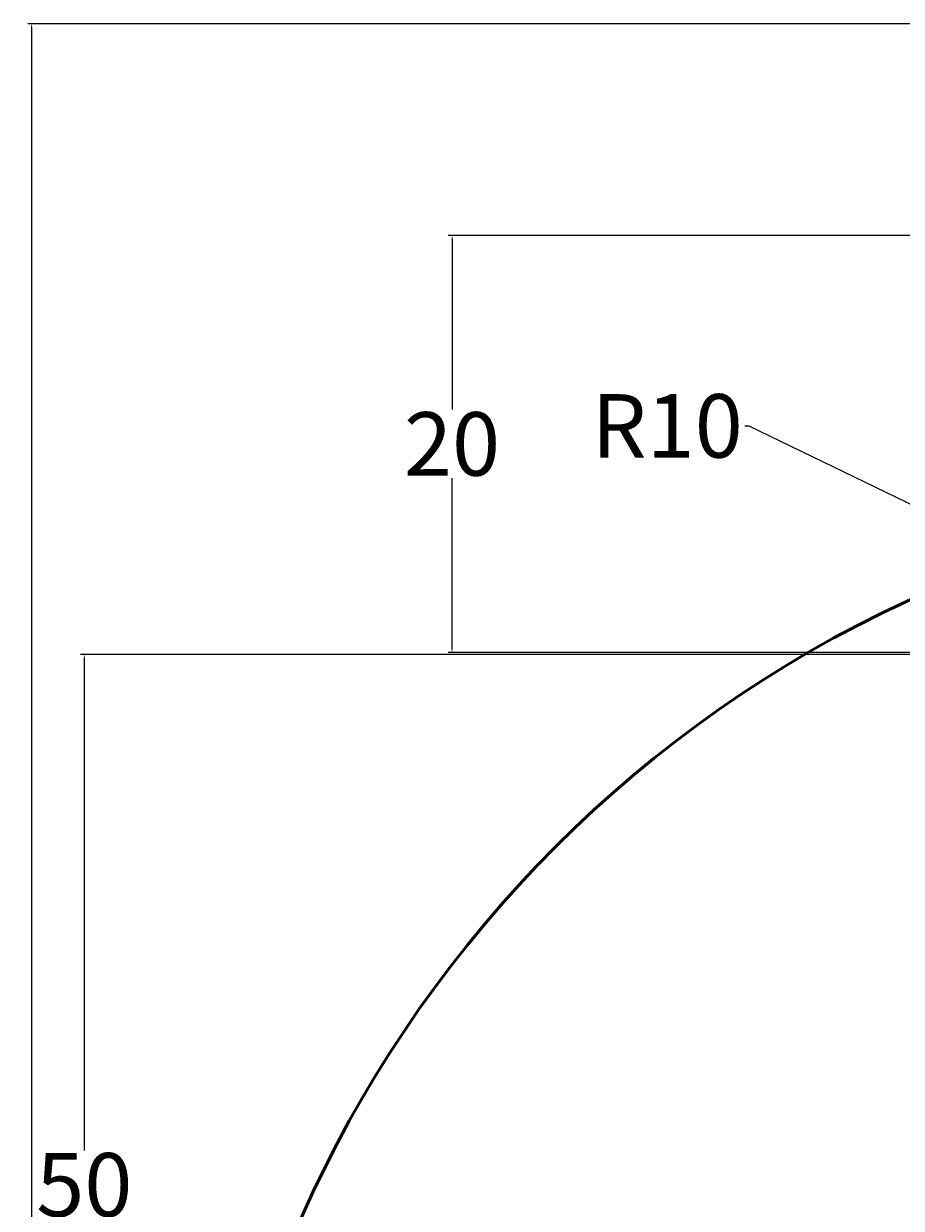
# Model space of a CAD drawing. Units: millimetres. Extents: x -53 to 92, y -147 to 37.
# Tile 10 of 16: x -47 to -6, y -30 to 26. Entities that reach past the tile are written whole.
import ezdxf

# ---------------------------------------------------------------- set-up
doc = ezdxf.new("R2010")
doc.units = ezdxf.units.MM
doc.header["$MEASUREMENT"] = 0
doc.layers.add('M-DIMS', color=2, linetype='Continuous', lineweight=25)
doc.layers.add('M-OUTL', color=7, linetype='Continuous', lineweight=50)
doc.styles.get("Standard").update_dxf_attribs({"font": 'arial.ttf'})
doc.dimstyles.get("Standard").update_dxf_attribs({"dimtxt": 0.18, "dimasz": 0.18, "dimexe": 0.18, "dimexo": 0.0625, "dimgap": 0.09, "dimtad": 0, "dimtih": 1, "dimtoh": 1, "dimdec": 4, "dimzin": 0, "dimdsep": 46, "dimtxsty": 'Standard', "dimcen": 0.09, "dimadec": 0, "dimazin": 0, "dimtfac": 1, "dimtdec": 4, "dimtofl": 0, "dimtmove": 0, "dimatfit": 3, "dimfxl": 1, "dimtolj": 1, "dimtzin": 0, "dimarcsym": 0})

# ---------------------------------------------------------------- blocks, each defined once
blk = doc.blocks.new('*D2')
at = {"layer": 'Defpoints', "color": 0, "transparency": 16777216}
for p in [(0.354, 0.478), (9.355, -3.88)]:
    blk.add_point(p, dxfattribs=at)
at = {"layer": 'M-DIMS', "color": 0, "lineweight": -2, "transparency": 16777216}
for p, q in [((-13.114, 6.912), (-12.934, 6.912)), ((-12.934, 6.912), (0.192, 0.557)), ((9.265, -3.88), (9.445, -3.88)), ((9.355, -3.97), (9.355, -3.79))]:
    blk.add_line(p, q, dxfattribs=at)
at = {"layer": 'M-DIMS', "color": 0, "transparency": 16777216}
blk.add_solid([(0.205, 0.584), (0.179, 0.53), (0.354, 0.478)], dxfattribs=at)
at = {"layer": 'M-DIMS', "color": 0, "transparency": 16777216, "insert": (-16.783, 6.912), "char_height": 0.18, "attachment_point": 5}
blk.add_mtext('\\A1;{\\H16.66667x;R10}', dxfattribs=at)
blk = doc.blocks.new('*D6')
at = {"layer": 'Defpoints', "color": 0, "transparency": 16777216}
for p in [(-26.95, 15.91), (28.602, 15.91), (9.355, -3.79)]:
    blk.add_point(p, dxfattribs=at)
at = {"layer": 'M-DIMS', "color": 0, "lineweight": -2, "transparency": 16777216}
for p, q in [((28.539, 15.91), (-27.13, 15.91)), ((-26.95, 15.73), (-26.95, 7.682)), ((-26.95, -3.61), (-26.95, 4.438)), ((9.292, -3.79), (-27.13, -3.79))]:
    blk.add_line(p, q, dxfattribs=at)
at = {"layer": 'M-DIMS', "color": 0, "transparency": 16777216}
for points in [[(-26.98, 15.73), (-26.92, 15.73), (-26.95, 15.91)], [(-26.98, -3.61), (-26.92, -3.61), (-26.95, -3.79)]]:
    blk.add_solid(points, dxfattribs=at)
at = {"layer": 'M-DIMS', "color": 0, "transparency": 16777216, "insert": (-26.95, 6.06), "char_height": 0.18, "attachment_point": 5}
blk.add_mtext('\\A1;{\\H16.66667x;20}', dxfattribs=at)
blk = doc.blocks.new('*D7')
at = {"layer": 'Defpoints', "color": 0, "transparency": 16777216}
for p in [(9.445, -3.88), (-44.321, -53.98), (18.956, -53.98)]:
    blk.add_point(p, dxfattribs=at)
at = {"layer": 'M-DIMS', "color": 0, "lineweight": -2, "transparency": 16777216}
for p, q in [((9.382, -3.88), (-44.501, -3.88)), ((-44.321, -4.06), (-44.321, -27.308)), ((-44.321, -53.8), (-44.321, -30.552)), ((18.894, -53.98), (-44.501, -53.98))]:
    blk.add_line(p, q, dxfattribs=at)
at = {"layer": 'M-DIMS', "color": 0, "transparency": 16777216}
for points in [[(-44.351, -4.06), (-44.291, -4.06), (-44.321, -3.88)], [(-44.351, -53.8), (-44.291, -53.8), (-44.321, -53.98)]]:
    blk.add_solid(points, dxfattribs=at)
at = {"layer": 'M-DIMS', "color": 0, "transparency": 16777216, "insert": (-44.321, -28.93), "char_height": 0.18, "attachment_point": 5}
blk.add_mtext('\\A1;{\\H16.66667x;50}', dxfattribs=at)
blk = doc.blocks.new('*D10')
at = {"layer": 'Defpoints', "color": 0, "transparency": 16777216}
for p in [(64.593, -18.184), (-26.68, -89.776)]:
    blk.add_point(p, dxfattribs=at)
at = {"layer": 'M-DIMS', "color": 0, "lineweight": -2, "transparency": 16777216}
for p, q in [((77.384, -8.151), (64.734, -18.073)), ((77.564, -8.151), (77.384, -8.151)), ((18.866, -53.98), (19.046, -53.98)), ((18.956, -54.07), (18.956, -53.89))]:
    blk.add_line(p, q, dxfattribs=at)
at = {"layer": 'M-DIMS', "color": 0, "transparency": 16777216}
blk.add_solid([(64.716, -18.05), (64.753, -18.097), (64.593, -18.184)], dxfattribs=at)
at = {"layer": 'M-DIMS', "color": 0, "transparency": 16777216, "insert": (82.599, -8.151), "char_height": 0.18, "attachment_point": 5}
blk.add_mtext('\\A1;{\\H16.66667x;%%C116}', dxfattribs=at)
blk = doc.blocks.new('*D17')
at = {"layer": 'Defpoints', "color": 0, "transparency": 16777216}
for p in [(-46.81, 25.909), (28.564, 25.909), (18.165, -111.975)]:
    blk.add_point(p, dxfattribs=at)
at = {"layer": 'M-DIMS', "color": 0, "lineweight": -2, "transparency": 16777216}
for p, q in [((28.502, 25.909), (-46.99, 25.909)), ((-46.81, 25.729), (-46.81, -42.851)), ((-46.81, -111.795), (-46.81, -43.215)), ((18.102, -111.975), (-46.99, -111.975))]:
    blk.add_line(p, q, dxfattribs=at)
at = {"layer": 'M-DIMS', "color": 0, "transparency": 16777216}
for points in [[(-46.84, 25.729), (-46.78, 25.729), (-46.81, 25.909)], [(-46.84, -111.795), (-46.78, -111.795), (-46.81, -111.975)]]:
    blk.add_solid(points, dxfattribs=at)
at = {"layer": 'M-DIMS', "color": 0, "transparency": 16777216, "insert": (-46.81, -43.033), "char_height": 0.18, "attachment_point": 5}
blk.add_mtext('\\A1;137.88', dxfattribs=at)

msp = doc.modelspace()

# ---------------------------------------------------------------- linework, layer by layer
at = {"layer": 'M-OUTL'}
msp.add_arc((18.95638, -53.98007), 58, 108.3895553, 70.0459142, dxfattribs=at)

# ---------------------------------------------------------------- dimensions: what is measured, and where the dimension line sits
at = {"layer": 'M-DIMS'}
dim = msp.add_linear_dim(base=(-46.8103, 25.90924), p1=(18.16452, -111.97467), p2=(28.56407, 25.90924), angle=90, dimstyle='Standard', override={"dimdec": 2, "dimlfac": 1, "dimrnd": 0, "dimzin": 0, "dimdsep": 46, "dimlunit": 2}, dxfattribs=at)
dim.commit()
dim.dimension.update_dxf_attribs({"geometry": '*D17', "text_midpoint": (-46.8103, -43.03271)})
for base, p1, p2, text, picture, middle in [((-26.95014, 15.91006), (9.35461, -3.78977), (28.60189, 15.91006), '{\\H16.66667x;20}', '*D6', (-26.95014, 6.06014)), ((-44.32095, -53.98007), (9.44461, -3.87977), (18.95638, -53.98007), '{\\H16.66667x;50}', '*D7', (-44.32095, -28.92992))]:
    dim = msp.add_linear_dim(base=base, p1=p1, p2=p2, angle=90, text=text, dimstyle='Standard', override={"dimclrd": 0, "dimclre": 0, "dimclrt": 0}, dxfattribs=at)
    dim.commit()
    dim.dimension.update_dxf_attribs({"geometry": picture, "text_midpoint": middle})
dim = msp.add_radius_dim(center=(9.35461, -3.87977), mpoint=(0.35416, 0.47819), text='{\\H16.66667x;R10}', dimstyle='Standard', override={"dimclrd": 0, "dimclre": 0, "dimclrt": 0}, dxfattribs=at)
dim.commit()
dim.dimension.update_dxf_attribs({"geometry": '*D2', "text_midpoint": (-16.78265, 6.912), "dimtype": 164})
dim = msp.add_diameter_dim_2p(p1=(-26.67986, -89.77579), p2=(64.59262, -18.18435), text='{\\H16.66667x;%%C116}', dimstyle='Standard', override={"dimclrd": 0, "dimclre": 0, "dimclrt": 0}, dxfattribs=at)
dim.commit()
dim.dimension.update_dxf_attribs({"geometry": '*D10', "text_midpoint": (82.59889, -8.15132), "dimtype": 163})

doc.saveas('drawing.dxf')
